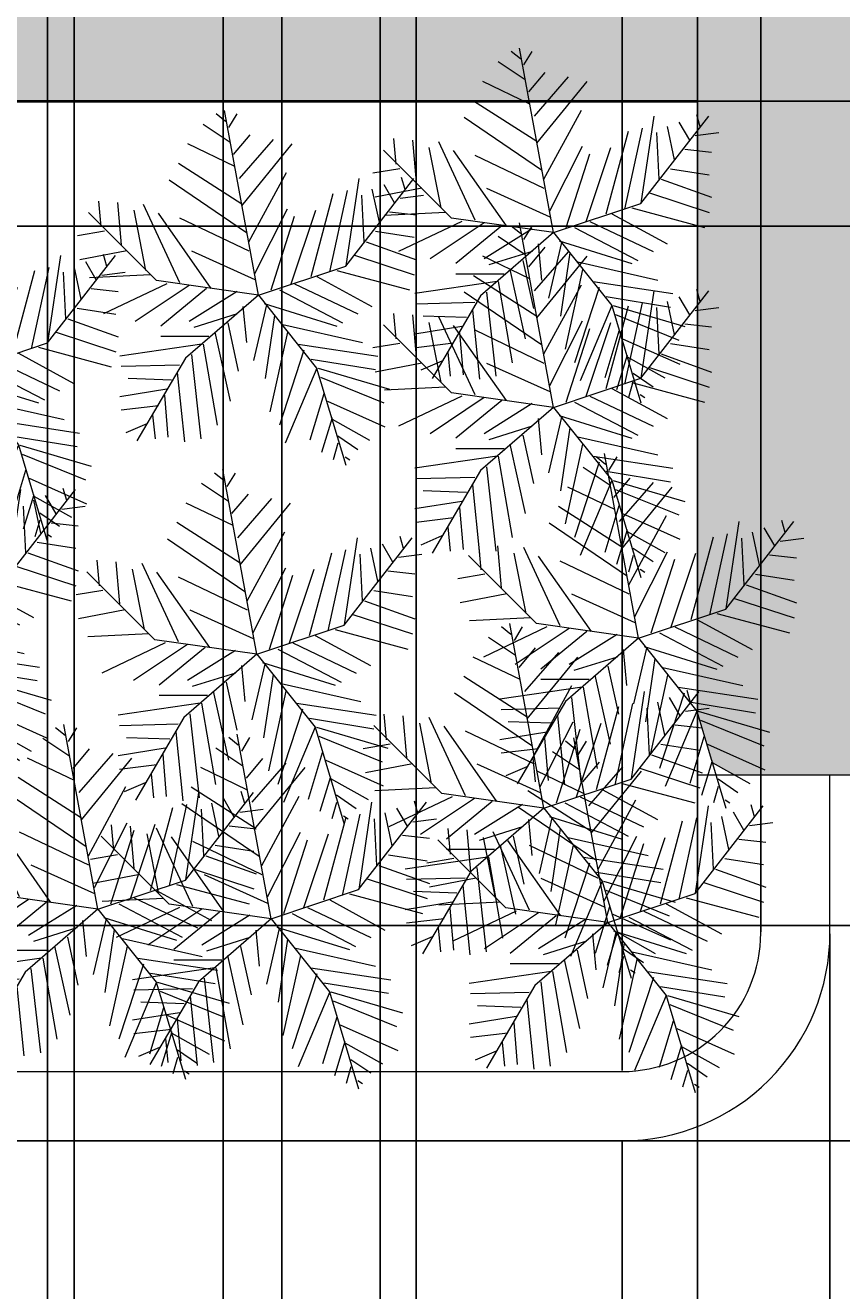
# Model space of a CAD drawing. Units: inches. Extents: x 818 to 1898, y 976 to 2364.
# Tile 40 of 96: x 1667 to 1714, y 1277 to 1350. Entities that reach past the tile are written whole.
import ezdxf

# ---------------------------------------------------------------- set-up
doc = ezdxf.new("R2010")
doc.units = ezdxf.units.IN
doc.header["$LTSCALE"] = 5
doc.header["$MEASUREMENT"] = 0
for name, color, linetype, lineweight in [('A-ANNO-DIMS', 2, 'Continuous', 18), ('A-WALL', 7, 'Continuous', 40), ('L-PLNT-BEDS', 94, 'Continuous', 18)]:
    doc.layers.add(name, color=color, linetype=linetype, lineweight=lineweight)
doc.layers.add('A-WALL-PATT', color=251, linetype='Continuous', lineweight=13, true_color=0x636466)
doc.layers.add('L-PLNT', color=116, linetype='Continuous', lineweight=13, true_color=0x136734)
doc.styles.get("Standard").update_dxf_attribs({"font": 'arial.ttf'})
doc.dimstyles.get("Standard").update_dxf_attribs({"dimtxt": 0.18, "dimasz": 0.18, "dimexe": 0.18, "dimexo": 0.0625, "dimgap": 0.09, "dimtad": 0, "dimtih": 1, "dimtoh": 1, "dimdec": 4, "dimzin": 0, "dimdsep": 46, "dimtxsty": 'Standard', "dimcen": 0.09, "dimadec": 0, "dimazin": 0, "dimtfac": 1, "dimtdec": 4, "dimtofl": 0, "dimtmove": 0, "dimatfit": 3, "dimfxl": 1, "dimtolj": 1, "dimtzin": 0, "dimarcsym": 0})

# ---------------------------------------------------------------- blocks, each defined once
blk = doc.blocks.new('SHRUB-ACCENT')
for p, q in [((10.438, 9.815), (8.475, 20.472)), ((8.533, 19.844), (7.992, 20.278)), ((8.737, 19.496), (9.211, 20.278)), ((8.804, 18.628), (7.247, 19.67)), ((9.008, 17.934), (9.956, 19.062)), ((9.075, 17.239), (6.366, 18.541)), ((9.346, 16.544), (11.31, 18.802)), ((9.482, 14.981), (12.394, 18.541)), ((9.482, 15.068), (5.824, 17.413)), ((9.888, 12.898), (12.055, 16.892)), ((9.753, 13.419), (5.283, 16.458)), ((15.486, 11.498), (19.412, 16.546)), ((15.509, 11.509), (16.254, 16.544)), ((17.677, 16.197), (18.286, 15.155)), ((18.693, 16.631), (18.896, 15.937)), ((13.478, 10.901), (14.764, 15.676)), ((14.561, 11.161), (15.577, 15.85)), ((16.39, 15.589), (16.525, 12.898)), ((16.999, 15.937), (17.406, 14.026)), ((18.625, 15.416), (19.979, 15.589)), ((1.354, 13.766), (1.219, 15.242)), ((2.303, 15.155), (2.506, 12.724)), ((3.251, 14.721), (3.928, 11.248)), ((3.793, 15.068), (5.892, 10.553)), ((10.227, 11.074), (12.123, 14.808)), ((12.326, 10.467), (13.748, 14.721)), ((18.015, 14.634), (19.573, 14.461)), ((4.549, 10.657), (0.623, 14.583)), ((7.721, 10.206), (4.673, 14.547)), ((5.892, 14.287), (9.888, 12.377)), ((11.175, 10.119), (12.529, 14.374)), ((1.558, 13.505), (0, 13.245)), ((17.203, 13.505), (19.437, 13.158)), ((16.661, 12.898), (19.573, 11.856)), ((2.845, 12.377), (0.136, 11.856)), ((6.569, 12.377), (10.227, 10.727)), ((15.983, 12.116), (19.437, 10.988)), ((4.199, 10.988), (0.677, 10.814)), ((10.438, 9.815), (15.486, 11.498)), ((14.968, 11.248), (19.166, 10.119)), ((5.147, 10.467), (1.49, 8.73)), ((6.434, 10.38), (3.319, 8.296)), ((10.438, 9.815), (4.549, 10.657)), ((12.529, 10.467), (16.187, 8.73)), ((13.816, 10.901), (16.999, 9.164)), ((7.45, 10.206), (4.809, 8.035)), ((10.438, 9.815), (6.231, 6.17)), ((9.211, 10.033), (6.434, 8.296)), ((10.438, 9.815), (13.803, 5.609)), ((11.649, 10.119), (15.306, 8.209)), ((9.549, 9.164), (9.753, 7.08)), ((10.904, 9.251), (10.159, 6.039)), ((10.769, 9.338), (14.968, 8.035)), ((9.211, 8.73), (6.705, 7.949)), ((8.669, 8.209), (9.278, 5.431)), ((11.378, 8.643), (10.836, 4.997)), ((11.852, 8.122), (16.457, 7.08)), ((7.585, 7.428), (4.809, 7.428)), ((7.924, 7.688), (8.804, 3.694)), ((12.123, 7.688), (11.107, 3.086)), ((7.179, 6.994), (2.438, 6.299)), ((7.247, 6.994), (8.06, 2.305)), ((13.071, 6.646), (11.649, 2.305)), ((12.733, 6.994), (17.338, 6.299)), ((6.231, 6.17), (3.427, 1.402)), ((6.569, 6.386), (7.111, 1.524)), ((13.478, 6.125), (17.203, 5.517)), ((5.892, 5.778), (2.506, 5.691)), ((5.757, 5.344), (6.163, 1.35)), ((13.816, 5.604), (11.988, 1.263)), ((13.803, 5.609), (15.486, 0)), ((13.884, 5.604), (18.015, 4.389)), ((5.147, 4.389), (2.438, 3.955)), ((5.418, 4.91), (2.912, 4.997)), ((14.019, 5.083), (17.677, 3.607)), ((5.012, 4.041), (5.215, 1.61)), ((14.223, 4.128), (13.41, 1.437)), ((14.426, 3.694), (17.744, 2.218)), ((4.673, 3.434), (2.506, 3.173)), ((3.996, 2.392), (2.777, 1.871)), ((4.334, 2.913), (4.47, 1.524)), ((14.697, 2.739), (14.087, 0.742)), ((14.697, 2.652), (16.864, 1.437)), ((15.035, 1.697), (16.187, 0.916)), ((15.035, 1.263), (14.764, 0.308)), ((15.442, 0.482), (15.712, 0.308))]:
    blk.add_line(p, q)
blk = doc.blocks.new('*D65')
at = {"layer": 'A-ANNO-DIMS', "color": 0, "lineweight": -2, "ltscale": 5, "transparency": 16777216}
for p, q in [((1430.725, 1346.016), (1430.725, 975.663)), ((1714.725, 1346.016), (1714.725, 975.663)), ((1430.905, 975.843), (1572.435, 975.843)), ((1714.545, 975.843), (1573.015, 975.843))]:
    blk.add_line(p, q, dxfattribs=at)
at = {"layer": 'A-ANNO-DIMS', "color": 0, "ltscale": 5, "transparency": 16777216}
for points in [[(1430.905, 975.873), (1430.905, 975.813), (1430.725, 975.843)], [(1714.545, 975.873), (1714.545, 975.813), (1714.725, 975.843)]]:
    blk.add_solid(points, dxfattribs=at)
at = {"layer": 'Defpoints', "color": 0, "ltscale": 5, "transparency": 16777216}
for p in [(1430.725, 1346.078), (1714.725, 1346.078), (1714.725, 975.843)]:
    blk.add_point(p, dxfattribs=at)
at = {"layer": 'A-ANNO-DIMS', "color": 0, "ltscale": 5, "transparency": 16777216, "insert": (1572.725, 975.843), "char_height": 0.18, "attachment_point": 5}
blk.add_mtext('\\A1;284', dxfattribs=at)
blk = doc.blocks.new('*D103')
at = {"layer": 'A-ANNO-DIMS', "color": 0, "lineweight": -2, "ltscale": 5, "transparency": 16777216}
for p, q in [((1626.575, 1071.118), (1626.575, 2363.873)), ((1626.755, 2363.693), (1657.699, 2363.693)), ((1689.291, 2363.693), (1658.348, 2363.693)), ((1689.471, 1071.118), (1689.471, 2363.873))]:
    blk.add_line(p, q, dxfattribs=at)
at = {"layer": 'A-ANNO-DIMS', "color": 0, "ltscale": 5, "transparency": 16777216}
for points in [[(1626.755, 2363.723), (1626.755, 2363.663), (1626.575, 2363.693)], [(1689.291, 2363.723), (1689.291, 2363.663), (1689.471, 2363.693)]]:
    blk.add_solid(points, dxfattribs=at)
at = {"layer": 'Defpoints', "color": 0, "ltscale": 5, "transparency": 16777216}
for p in [(1689.471, 2363.693), (1626.575, 1071.055), (1689.471, 1071.055)]:
    blk.add_point(p, dxfattribs=at)
at = {"layer": 'A-ANNO-DIMS', "color": 0, "ltscale": 5, "transparency": 16777216, "insert": (1658.023, 2363.693), "char_height": 0.18, "attachment_point": 5}
blk.add_mtext('\\A1;62.9', dxfattribs=at)
blk = doc.blocks.new('*D104')
at = {"layer": 'A-ANNO-DIMS', "color": 0, "lineweight": -2, "ltscale": 5, "transparency": 16777216}
for p, q in [((1689.471, 1071.118), (1689.471, 2363.873)), ((1689.651, 2363.693), (1717.401, 2363.693)), ((1745.903, 2363.693), (1718.154, 2363.693)), ((1746.083, 1071.118), (1746.083, 2363.873))]:
    blk.add_line(p, q, dxfattribs=at)
at = {"layer": 'A-ANNO-DIMS', "color": 0, "ltscale": 5, "transparency": 16777216}
for points in [[(1689.651, 2363.723), (1689.651, 2363.663), (1689.471, 2363.693)], [(1745.903, 2363.723), (1745.903, 2363.663), (1746.083, 2363.693)]]:
    blk.add_solid(points, dxfattribs=at)
at = {"layer": 'Defpoints', "color": 0, "ltscale": 5, "transparency": 16777216}
for p in [(1746.083, 2363.693), (1689.471, 1071.055), (1746.083, 1071.055)]:
    blk.add_point(p, dxfattribs=at)
at = {"layer": 'A-ANNO-DIMS', "color": 0, "ltscale": 5, "transparency": 16777216, "insert": (1717.777, 2363.693), "char_height": 0.18, "attachment_point": 5}
blk.add_mtext('\\A1;56.61', dxfattribs=at)
blk = doc.blocks.new('*D113')
at = {"layer": 'A-ANNO-DIMS', "color": 0, "lineweight": -2, "ltscale": 5, "transparency": 16777216}
for p, q in [((1430.788, 1346.078), (1897.916, 1346.078)), ((1897.736, 1345.898), (1897.736, 1316.26)), ((1897.736, 1286.258), (1897.736, 1315.896)), ((1430.788, 1286.078), (1897.916, 1286.078))]:
    blk.add_line(p, q, dxfattribs=at)
at = {"layer": 'A-ANNO-DIMS', "color": 0, "ltscale": 5, "transparency": 16777216}
for points in [[(1897.706, 1345.898), (1897.766, 1345.898), (1897.736, 1346.078)], [(1897.706, 1286.258), (1897.766, 1286.258), (1897.736, 1286.078)]]:
    blk.add_solid(points, dxfattribs=at)
at = {"layer": 'Defpoints', "color": 0, "ltscale": 5, "transparency": 16777216}
for p in [(1430.725, 1346.078), (1897.736, 1346.078), (1430.725, 1286.078)]:
    blk.add_point(p, dxfattribs=at)
at = {"layer": 'A-ANNO-DIMS', "color": 0, "ltscale": 5, "transparency": 16777216, "insert": (1897.736, 1316.078), "char_height": 0.18, "attachment_point": 5}
blk.add_mtext('\\A1;60', dxfattribs=at)
blk = doc.blocks.new('*D115')
at = {"layer": 'A-ANNO-DIMS', "color": 0, "lineweight": -2, "ltscale": 5, "transparency": 16777216}
for p, q in [((1766.29, 1377.656), (818.026, 1377.656)), ((818.206, 1377.476), (818.206, 1338.262)), ((818.206, 1298.684), (818.206, 1337.898)), ((1766.29, 1298.504), (818.026, 1298.504))]:
    blk.add_line(p, q, dxfattribs=at)
at = {"layer": 'A-ANNO-DIMS', "color": 0, "ltscale": 5, "transparency": 16777216}
for points in [[(818.176, 1377.476), (818.236, 1377.476), (818.206, 1377.656)], [(818.176, 1298.684), (818.236, 1298.684), (818.206, 1298.504)]]:
    blk.add_solid(points, dxfattribs=at)
at = {"layer": 'Defpoints', "color": 0, "ltscale": 5, "transparency": 16777216}
for p in [(818.206, 1377.656), (1766.352, 1377.656), (1766.352, 1298.504)]:
    blk.add_point(p, dxfattribs=at)
at = {"layer": 'A-ANNO-DIMS', "color": 0, "ltscale": 5, "transparency": 16777216, "insert": (818.206, 1338.08), "char_height": 0.18, "attachment_point": 5}
blk.add_mtext('\\A1;79.15', dxfattribs=at)
blk = doc.blocks.new('*D153')
at = {"layer": 'A-ANNO-DIMS', "color": 0, "lineweight": -2, "ltscale": 5, "transparency": 16777216}
for p, q in [((1713.369, 1298.016), (1713.369, 975.663)), ((1701.369, 1286.016), (1701.369, 975.663)), ((1701.549, 975.843), (1707.159, 975.843)), ((1713.189, 975.843), (1707.578, 975.843))]:
    blk.add_line(p, q, dxfattribs=at)
at = {"layer": 'A-ANNO-DIMS', "color": 0, "ltscale": 5, "transparency": 16777216}
for points in [[(1701.549, 975.873), (1701.549, 975.813), (1701.369, 975.843)], [(1713.189, 975.873), (1713.189, 975.813), (1713.369, 975.843)]]:
    blk.add_solid(points, dxfattribs=at)
at = {"layer": 'Defpoints', "color": 0, "ltscale": 5, "transparency": 16777216}
for p in [(1713.369, 1298.078), (1701.369, 1286.078), (1713.369, 975.843)]:
    blk.add_point(p, dxfattribs=at)
at = {"layer": 'A-ANNO-DIMS', "color": 0, "ltscale": 5, "transparency": 16777216, "insert": (1707.369, 975.843), "char_height": 0.18, "attachment_point": 5}
blk.add_mtext('\\A1;12', dxfattribs=at)
blk = doc.blocks.new('*D154')
at = {"layer": 'A-ANNO-DIMS', "color": 0, "lineweight": -2, "ltscale": 5, "transparency": 16777216}
for p, q in [((1701.369, 1290.141), (1701.369, 2363.873)), ((1701.549, 2363.693), (1705.22, 2363.693)), ((1709.189, 2363.693), (1705.518, 2363.693)), ((1709.369, 1298.141), (1709.369, 2363.873))]:
    blk.add_line(p, q, dxfattribs=at)
at = {"layer": 'A-ANNO-DIMS', "color": 0, "ltscale": 5, "transparency": 16777216}
for points in [[(1701.549, 2363.723), (1701.549, 2363.663), (1701.369, 2363.693)], [(1709.189, 2363.723), (1709.189, 2363.663), (1709.369, 2363.693)]]:
    blk.add_solid(points, dxfattribs=at)
at = {"layer": 'Defpoints', "color": 0, "ltscale": 5, "transparency": 16777216}
for p in [(1709.369, 2363.693), (1709.369, 1298.078), (1701.369, 1290.078)]:
    blk.add_point(p, dxfattribs=at)
at = {"layer": 'A-ANNO-DIMS', "color": 0, "ltscale": 5, "transparency": 16777216, "insert": (1705.369, 2363.693), "char_height": 0.18, "attachment_point": 5}
blk.add_mtext('\\A1;8', dxfattribs=at)
blk = doc.blocks.new('*D178')
at = {"layer": 'A-ANNO-DIMS', "color": 0, "lineweight": -2, "ltscale": 5, "transparency": 16777216}
for p, q in [((1669.725, 1600.016), (1669.725, 975.663)), ((1705.725, 1600.016), (1705.725, 975.663)), ((1669.905, 975.843), (1687.506, 975.843)), ((1705.545, 975.843), (1687.944, 975.843))]:
    blk.add_line(p, q, dxfattribs=at)
at = {"layer": 'A-ANNO-DIMS', "color": 0, "ltscale": 5, "transparency": 16777216}
for points in [[(1669.905, 975.873), (1669.905, 975.813), (1669.725, 975.843)], [(1705.545, 975.873), (1705.545, 975.813), (1705.725, 975.843)]]:
    blk.add_solid(points, dxfattribs=at)
at = {"layer": 'Defpoints', "color": 0, "ltscale": 5, "transparency": 16777216}
for p in [(1669.725, 1600.078), (1705.725, 1600.078), (1705.725, 975.843)]:
    blk.add_point(p, dxfattribs=at)
at = {"layer": 'A-ANNO-DIMS', "color": 0, "ltscale": 5, "transparency": 16777216, "insert": (1687.725, 975.843), "char_height": 0.18, "attachment_point": 5}
blk.add_mtext('\\A1;36', dxfattribs=at)
blk = doc.blocks.new('*D180')
at = {"layer": 'A-ANNO-DIMS', "color": 0, "lineweight": -2, "ltscale": 5, "transparency": 16777216}
for p, q in [((1599.725, 1639.516), (1599.725, 975.663)), ((1669.725, 1639.516), (1669.725, 975.663)), ((1599.905, 975.843), (1634.507, 975.843)), ((1669.545, 975.843), (1634.943, 975.843))]:
    blk.add_line(p, q, dxfattribs=at)
at = {"layer": 'A-ANNO-DIMS', "color": 0, "ltscale": 5, "transparency": 16777216}
for points in [[(1599.905, 975.873), (1599.905, 975.813), (1599.725, 975.843)], [(1669.545, 975.873), (1669.545, 975.813), (1669.725, 975.843)]]:
    blk.add_solid(points, dxfattribs=at)
at = {"layer": 'Defpoints', "color": 0, "ltscale": 5, "transparency": 16777216}
for p in [(1599.725, 1639.578), (1669.725, 1639.578), (1669.725, 975.843)]:
    blk.add_point(p, dxfattribs=at)
at = {"layer": 'A-ANNO-DIMS', "color": 0, "ltscale": 5, "transparency": 16777216, "insert": (1634.725, 975.843), "char_height": 0.18, "attachment_point": 5}
blk.add_mtext('\\A1;70', dxfattribs=at)
blk = doc.blocks.new('*D193')
at = {"layer": 'A-ANNO-DIMS', "color": 0, "lineweight": -2, "ltscale": 5, "transparency": 16777216}
for p, q in [((1660.377, 1346.078), (1897.916, 1346.078)), ((1897.736, 1345.898), (1897.736, 1342.654)), ((1897.736, 1339.045), (1897.736, 1342.29)), ((1660.377, 1338.865), (1897.916, 1338.865))]:
    blk.add_line(p, q, dxfattribs=at)
at = {"layer": 'A-ANNO-DIMS', "color": 0, "ltscale": 5, "transparency": 16777216}
for points in [[(1897.706, 1345.898), (1897.766, 1345.898), (1897.736, 1346.078)], [(1897.706, 1339.045), (1897.766, 1339.045), (1897.736, 1338.865)]]:
    blk.add_solid(points, dxfattribs=at)
at = {"layer": 'Defpoints', "color": 0, "ltscale": 5, "transparency": 16777216}
for p in [(1660.314, 1346.078), (1897.736, 1346.078), (1660.314, 1338.865)]:
    blk.add_point(p, dxfattribs=at)
at = {"layer": 'A-ANNO-DIMS', "color": 0, "ltscale": 5, "transparency": 16777216, "insert": (1897.736, 1342.472), "char_height": 0.18, "attachment_point": 5}
blk.add_mtext('\\A1;7.213', dxfattribs=at)
blk = doc.blocks.new('*D198')
at = {"layer": 'A-ANNO-DIMS', "color": 0, "lineweight": -2, "ltscale": 5, "transparency": 16777216}
for p, q in [((1741.841, 1545.016), (1741.841, 975.663)), ((1430.725, 1346.016), (1430.725, 975.663)), ((1430.905, 975.843), (1585.907, 975.843)), ((1741.661, 975.843), (1586.659, 975.843))]:
    blk.add_line(p, q, dxfattribs=at)
at = {"layer": 'A-ANNO-DIMS', "color": 0, "ltscale": 5, "transparency": 16777216}
for points in [[(1430.905, 975.873), (1430.905, 975.813), (1430.725, 975.843)], [(1741.661, 975.873), (1741.661, 975.813), (1741.841, 975.843)]]:
    blk.add_solid(points, dxfattribs=at)
at = {"layer": 'Defpoints', "color": 0, "ltscale": 5, "transparency": 16777216}
for p in [(1741.841, 1545.078), (1430.725, 1346.078), (1741.841, 975.843)]:
    blk.add_point(p, dxfattribs=at)
at = {"layer": 'A-ANNO-DIMS', "color": 0, "ltscale": 5, "transparency": 16777216, "insert": (1586.283, 975.843), "char_height": 0.18, "attachment_point": 5}
blk.add_mtext('\\A1;311.1', dxfattribs=at)
blk = doc.blocks.new('*D199')
at = {"layer": 'A-ANNO-DIMS', "color": 0, "lineweight": -2, "ltscale": 5, "transparency": 16777216}
for p, q in [((1559.788, 1687.078), (1897.916, 1687.078)), ((1897.736, 1686.898), (1897.736, 1513.154)), ((1897.736, 1339.045), (1897.736, 1512.79)), ((1660.377, 1338.865), (1897.916, 1338.865))]:
    blk.add_line(p, q, dxfattribs=at)
at = {"layer": 'A-ANNO-DIMS', "color": 0, "ltscale": 5, "transparency": 16777216}
for points in [[(1897.706, 1686.898), (1897.766, 1686.898), (1897.736, 1687.078)], [(1897.706, 1339.045), (1897.766, 1339.045), (1897.736, 1338.865)]]:
    blk.add_solid(points, dxfattribs=at)
at = {"layer": 'Defpoints', "color": 0, "ltscale": 5, "transparency": 16777216}
for p in [(1559.725, 1687.078), (1897.736, 1687.078), (1660.314, 1338.865)]:
    blk.add_point(p, dxfattribs=at)
at = {"layer": 'A-ANNO-DIMS', "color": 0, "ltscale": 5, "transparency": 16777216, "insert": (1897.736, 1512.972), "char_height": 0.18, "attachment_point": 5}
blk.add_mtext('\\A1;348.2', dxfattribs=at)
blk = doc.blocks.new('*D200')
at = {"layer": 'A-ANNO-DIMS', "color": 0, "lineweight": -2, "ltscale": 5, "transparency": 16777216}
for p, q in [((1678.33, 1477.364), (1678.33, 975.663)), ((1705.725, 1477.364), (1705.725, 975.663)), ((1678.51, 975.843), (1691.562, 975.843)), ((1705.545, 975.843), (1692.493, 975.843))]:
    blk.add_line(p, q, dxfattribs=at)
at = {"layer": 'A-ANNO-DIMS', "color": 0, "ltscale": 5, "transparency": 16777216}
for points in [[(1678.51, 975.873), (1678.51, 975.813), (1678.33, 975.843)], [(1705.545, 975.873), (1705.545, 975.813), (1705.725, 975.843)]]:
    blk.add_solid(points, dxfattribs=at)
at = {"layer": 'Defpoints', "color": 0, "ltscale": 5, "transparency": 16777216}
for p in [(1678.33, 1477.426), (1705.725, 1477.426), (1705.725, 975.843)]:
    blk.add_point(p, dxfattribs=at)
at = {"layer": 'A-ANNO-DIMS', "color": 0, "ltscale": 5, "transparency": 16777216, "insert": (1692.028, 975.843), "char_height": 0.18, "attachment_point": 5}
blk.add_mtext('\\A1;27.395', dxfattribs=at)
blk = doc.blocks.new('*D212')
at = {"layer": 'A-ANNO-DIMS', "color": 0, "lineweight": -2, "ltscale": 5, "transparency": 16777216}
for p, q in [((1681.725, 1900.016), (1681.725, 975.663)), ((1705.725, 1876.016), (1705.725, 975.663)), ((1681.905, 975.843), (1693.505, 975.843)), ((1705.545, 975.843), (1693.945, 975.843))]:
    blk.add_line(p, q, dxfattribs=at)
at = {"layer": 'A-ANNO-DIMS', "color": 0, "ltscale": 5, "transparency": 16777216}
for points in [[(1681.905, 975.873), (1681.905, 975.813), (1681.725, 975.843)], [(1705.545, 975.873), (1705.545, 975.813), (1705.725, 975.843)]]:
    blk.add_solid(points, dxfattribs=at)
at = {"layer": 'Defpoints', "color": 0, "ltscale": 5, "transparency": 16777216}
for p in [(1681.725, 1900.078), (1705.725, 1876.078), (1705.725, 975.843)]:
    blk.add_point(p, dxfattribs=at)
at = {"layer": 'A-ANNO-DIMS', "color": 0, "ltscale": 5, "transparency": 16777216, "insert": (1693.725, 975.843), "char_height": 0.18, "attachment_point": 5}
blk.add_mtext('\\A1;24', dxfattribs=at)
blk = doc.blocks.new('*D214')
at = {"layer": 'A-ANNO-DIMS', "color": 0, "lineweight": -2, "ltscale": 5, "transparency": 16777216}
for p, q in [((1511.725, 1687.016), (1511.725, 975.663)), ((1714.725, 1687.016), (1714.725, 975.663)), ((1511.905, 975.843), (1612.935, 975.843)), ((1714.545, 975.843), (1613.516, 975.843))]:
    blk.add_line(p, q, dxfattribs=at)
at = {"layer": 'A-ANNO-DIMS', "color": 0, "ltscale": 5, "transparency": 16777216}
for points in [[(1511.905, 975.873), (1511.905, 975.813), (1511.725, 975.843)], [(1714.545, 975.873), (1714.545, 975.813), (1714.725, 975.843)]]:
    blk.add_solid(points, dxfattribs=at)
at = {"layer": 'Defpoints', "color": 0, "ltscale": 5, "transparency": 16777216}
for p in [(1511.725, 1687.078), (1714.725, 1687.078), (1714.725, 975.843)]:
    blk.add_point(p, dxfattribs=at)
at = {"layer": 'A-ANNO-DIMS', "color": 0, "ltscale": 5, "transparency": 16777216, "insert": (1613.225, 975.843), "char_height": 0.18, "attachment_point": 5}
blk.add_mtext('\\A1;203', dxfattribs=at)
blk = doc.blocks.new('*D221')
at = {"layer": 'A-ANNO-DIMS', "color": 0, "lineweight": -2, "ltscale": 5, "transparency": 16777216}
for p, q in [((1668.184, 1696.016), (1668.184, 975.663)), ((1705.725, 1696.016), (1705.725, 975.663)), ((1668.364, 975.843), (1686.561, 975.843)), ((1705.545, 975.843), (1687.348, 975.843))]:
    blk.add_line(p, q, dxfattribs=at)
at = {"layer": 'A-ANNO-DIMS', "color": 0, "ltscale": 5, "transparency": 16777216}
for points in [[(1668.364, 975.873), (1668.364, 975.813), (1668.184, 975.843)], [(1705.545, 975.873), (1705.545, 975.813), (1705.725, 975.843)]]:
    blk.add_solid(points, dxfattribs=at)
at = {"layer": 'Defpoints', "color": 0, "ltscale": 5, "transparency": 16777216}
for p in [(1668.184, 1696.078), (1705.725, 1696.078), (1705.725, 975.843)]:
    blk.add_point(p, dxfattribs=at)
at = {"layer": 'A-ANNO-DIMS', "color": 0, "ltscale": 5, "transparency": 16777216, "insert": (1686.955, 975.843), "char_height": 0.18, "attachment_point": 5}
blk.add_mtext('\\A1;37.54', dxfattribs=at)
blk = doc.blocks.new('*D228')
at = {"layer": 'A-ANNO-DIMS', "color": 0, "lineweight": -2, "ltscale": 5, "transparency": 16777216}
for p, q in [((1687.394, 1802.016), (1687.394, 975.663)), ((1705.725, 1802.016), (1705.725, 975.663)), ((1687.574, 975.843), (1696.174, 975.843)), ((1705.545, 975.843), (1696.945, 975.843))]:
    blk.add_line(p, q, dxfattribs=at)
at = {"layer": 'A-ANNO-DIMS', "color": 0, "ltscale": 5, "transparency": 16777216}
for points in [[(1687.574, 975.873), (1687.574, 975.813), (1687.394, 975.843)], [(1705.545, 975.873), (1705.545, 975.813), (1705.725, 975.843)]]:
    blk.add_solid(points, dxfattribs=at)
at = {"layer": 'Defpoints', "color": 0, "ltscale": 5, "transparency": 16777216}
for p in [(1687.394, 1802.078), (1705.725, 1802.078), (1705.725, 975.843)]:
    blk.add_point(p, dxfattribs=at)
at = {"layer": 'A-ANNO-DIMS', "color": 0, "ltscale": 5, "transparency": 16777216, "insert": (1696.56, 975.843), "char_height": 0.18, "attachment_point": 5}
blk.add_mtext('\\A1;18.33', dxfattribs=at)

msp = doc.modelspace()

# ---------------------------------------------------------------- hatches: boundary and pattern name
at = {"layer": 'A-WALL-PATT', "ltscale": 5}
h = msp.add_hatch(color=256, dxfattribs=at)
h.dxf.hatch_style = 1
h.paths.add_polyline_path([(1714.7251, 1521.0782), (1705.7251, 1521.0782), (1705.7251, 1467.0782), (1654.7252, 1467.0782), (1654.7252, 1463.0782), (1705.7251, 1463.0782), (1705.7251, 1355.0782), (1622.7252, 1355.0782), (1622.7252, 1379.0782), (1622.7252, 1386.6857), (1616.7252, 1386.6857), (1616.7252, 1355.0782), (1490.9163, 1355.0782), (1490.9163, 1346.0782), (1544.7605, 1346.0782), (1544.6132, 1346.8783), (1544.6729, 1346.84), (1544.6299, 1346.7874), (1544.7605, 1346.0782), (1555.1299, 1346.0782), (1555.1299, 1341.5528), (1556.1599, 1340.8639), (1556.5281, 1338.8654), (1660.3141, 1338.8654), (1660.3141, 1346.0782), (1705.7251, 1346.0782), (1705.7251, 1345.0768), (1705.8704, 1344.58), (1705.7251, 1344.3933), (1705.7251, 1334.9904), (1705.8704, 1334.4936), (1705.7251, 1334.3068), (1705.7251, 1316.2253), (1707.3573, 1316.7694), (1707.3847, 1316.8046), (1707.3807, 1316.7771), (1705.7251, 1316.2253), (1705.7251, 1314.1392), (1705.7251, 1312.0957), (1705.8703, 1312.0739), (1705.7251, 1311.8873), (1705.7251, 1310.7121), (1706.5603, 1307.9282), (1707.8887, 1307.1831), (1714.7251, 1307.1831), (1714.7251, 1346.0782)])

# ---------------------------------------------------------------- linework, layer by layer
at = {"layer": 'A-WALL'}
msp.add_line((1660.3141, 1346.0782), (1705.7251, 1346.0782), dxfattribs=at)
at = {"layer": 'L-PLNT'}
for p, q in [((1697.4011, 1338.4984), (1695.438, 1349.1549)), ((1695.7676, 1347.3112), (1694.2099, 1348.3531)), ((1695.4967, 1348.5268), (1694.9549, 1348.9609)), ((1695.6999, 1348.1794), (1696.1741, 1348.9609)), ((1695.9708, 1346.6166), (1696.9191, 1347.7453)), ((1696.0385, 1345.9219), (1693.3295, 1347.2242)), ((1696.3094, 1345.2273), (1698.2736, 1347.4848)), ((1696.445, 1343.6644), (1699.3572, 1347.2242)), ((1696.445, 1343.7513), (1692.7877, 1346.0956)), ((1696.8512, 1341.5805), (1699.0186, 1345.5747)), ((1696.7159, 1342.1016), (1692.2459, 1345.1404)), ((1702.4489, 1340.181), (1706.375, 1345.2288)), ((1702.4727, 1340.1914), (1703.2177, 1345.2273)), ((1704.6399, 1344.88), (1705.2494, 1343.8381)), ((1705.6558, 1345.3141), (1705.8588, 1344.6195)), ((1700.4408, 1339.5836), (1701.7276, 1344.3591)), ((1701.5244, 1339.8441), (1702.5403, 1344.5328)), ((1703.353, 1344.2722), (1703.4886, 1341.5805)), ((1703.9625, 1344.6195), (1704.369, 1342.7094)), ((1705.5881, 1344.0985), (1706.9426, 1344.2722)), ((1691.5119, 1339.3397), (1687.5858, 1343.2658)), ((1688.3177, 1342.449), (1688.1824, 1343.925)), ((1689.266, 1343.8381), (1689.469, 1341.407)), ((1690.214, 1343.4039), (1690.8914, 1339.931)), ((1690.7558, 1343.7513), (1692.8554, 1339.2363)), ((1694.684, 1338.8891), (1691.6364, 1343.2303)), ((1697.19, 1339.7573), (1699.0863, 1343.4909)), ((1699.2895, 1339.1495), (1700.7117, 1343.4039)), ((1704.9785, 1343.3172), (1706.5362, 1343.1435)), ((1692.8554, 1342.9698), (1696.8512, 1341.0597)), ((1698.138, 1338.8022), (1699.4926, 1343.0566)), ((1688.521, 1342.1883), (1686.9632, 1341.9279)), ((1704.1657, 1342.1883), (1706.4006, 1341.8412)), ((1689.8078, 1341.0597), (1687.0988, 1340.5386)), ((1693.5327, 1341.0597), (1697.19, 1339.41)), ((1703.6239, 1341.5805), (1706.5362, 1340.5386)), ((1702.9466, 1340.7992), (1706.4006, 1339.6704)), ((1691.1623, 1339.6704), (1687.6406, 1339.4967)), ((1697.4011, 1338.4984), (1702.4489, 1340.181)), ((1700.7794, 1339.5836), (1703.9625, 1337.8472)), ((1701.9309, 1339.931), (1706.1297, 1338.8022)), ((1692.1104, 1339.1495), (1688.4533, 1337.4131)), ((1693.3972, 1339.0626), (1690.2819, 1336.9788)), ((1697.4011, 1338.4984), (1691.5119, 1339.3397)), ((1694.4131, 1338.8891), (1691.7718, 1336.7183)), ((1695.4967, 1338.4403), (1694.9549, 1338.8744)), ((1697.4011, 1328.4119), (1695.438, 1339.0685)), ((1695.6999, 1338.093), (1696.1741, 1338.8744)), ((1699.4926, 1339.1495), (1703.1498, 1337.4131)), ((1697.4011, 1338.4984), (1693.1945, 1334.8527)), ((1696.1741, 1338.7154), (1693.3972, 1336.9788)), ((1695.7676, 1337.2247), (1694.2099, 1338.2666)), ((1697.4011, 1338.4984), (1700.7663, 1334.2918)), ((1698.6122, 1338.8022), (1702.2694, 1336.892)), ((1696.1741, 1337.4131), (1693.6681, 1336.6316)), ((1695.9708, 1336.5302), (1696.9191, 1337.6588)), ((1696.3094, 1335.1409), (1698.2736, 1337.3984)), ((1696.5126, 1337.8472), (1696.7159, 1335.7634)), ((1697.8671, 1337.9339), (1697.1223, 1334.7214)), ((1697.7318, 1338.0207), (1701.9309, 1336.7183)), ((1696.0385, 1335.8355), (1693.3295, 1337.1378)), ((1695.6323, 1336.892), (1696.2417, 1334.1136)), ((1696.445, 1333.5779), (1699.3572, 1337.1378)), ((1698.3413, 1337.3261), (1697.7995, 1333.6795)), ((1698.8154, 1336.8053), (1703.4207, 1335.7634)), ((1694.5487, 1336.1105), (1691.7718, 1336.1105)), ((1696.445, 1333.6649), (1692.7877, 1336.0091)), ((1694.8872, 1336.3712), (1695.7676, 1332.3772)), ((1699.0863, 1336.3712), (1698.0704, 1331.7694)), ((1694.1422, 1335.6764), (1689.4013, 1334.9819)), ((1694.2099, 1335.6764), (1695.0228, 1330.9879)), ((1696.8512, 1331.4941), (1699.0186, 1335.4883)), ((1700.0344, 1335.3292), (1698.6122, 1330.9879)), ((1699.6958, 1335.6764), (1704.3011, 1334.9819)), ((1705.6558, 1335.2277), (1705.8588, 1334.5331)), ((1692.8554, 1334.4608), (1689.469, 1334.3741)), ((1693.1945, 1334.8527), (1690.3902, 1330.0853)), ((1696.7159, 1332.0152), (1692.2459, 1335.054)), ((1693.5327, 1335.0686), (1694.0745, 1330.2064)), ((1700.4408, 1334.8082), (1704.1657, 1334.2004)), ((1701.5244, 1329.7576), (1702.5403, 1334.4464)), ((1702.4489, 1330.0945), (1706.375, 1335.1424)), ((1702.4727, 1330.105), (1703.2177, 1335.1409)), ((1703.9625, 1334.5331), (1704.369, 1332.623)), ((1704.6399, 1334.7935), (1705.2494, 1333.7516)), ((1688.3177, 1332.3625), (1688.1824, 1333.8386)), ((1689.266, 1333.7516), (1689.469, 1331.3206)), ((1692.72, 1334.0267), (1693.1263, 1330.0327)), ((1700.7794, 1334.2873), (1698.9508, 1329.946)), ((1700.4408, 1329.4972), (1701.7276, 1334.2727)), ((1700.7663, 1334.2918), (1702.4489, 1328.6831)), ((1700.8473, 1334.2873), (1704.9785, 1333.0717)), ((1700.9826, 1333.7663), (1704.6399, 1332.2902)), ((1703.353, 1334.1857), (1703.4886, 1331.4941)), ((1705.5881, 1334.0121), (1706.9426, 1334.1857)), ((1691.5119, 1329.2532), (1687.5858, 1333.1793)), ((1692.1104, 1333.0717), (1689.4013, 1332.6376)), ((1692.3814, 1333.5926), (1689.8755, 1333.6795)), ((1690.214, 1333.3175), (1690.8914, 1329.8446)), ((1690.7558, 1333.6649), (1692.8554, 1329.1499)), ((1694.684, 1328.8027), (1691.6364, 1333.1438)), ((1697.19, 1329.6709), (1699.0863, 1333.4044)), ((1698.138, 1328.7157), (1699.4926, 1332.9701)), ((1699.2895, 1329.0631), (1700.7117, 1333.3175)), ((1704.9785, 1333.2308), (1706.5362, 1333.0571)), ((1691.975, 1332.7244), (1692.1782, 1330.2934)), ((1692.8554, 1332.8834), (1696.8512, 1330.9732)), ((1701.1858, 1332.8113), (1700.3731, 1330.1197)), ((1701.3891, 1332.3772), (1704.7075, 1330.9012)), ((1688.521, 1332.1019), (1686.9632, 1331.8415)), ((1691.6364, 1332.1166), (1689.469, 1331.8561)), ((1691.2976, 1331.5957), (1691.4332, 1330.2064)), ((1704.1657, 1332.1019), (1706.4006, 1331.7547)), ((1689.8078, 1330.9732), (1687.0988, 1330.4522)), ((1690.9591, 1331.0746), (1689.7399, 1330.5538)), ((1693.5327, 1330.9732), (1697.19, 1329.3235)), ((1701.66, 1331.422), (1701.0503, 1329.4249)), ((1701.66, 1331.3353), (1703.8272, 1330.1197)), ((1703.6239, 1331.4941), (1706.5362, 1330.4522)), ((1697.4011, 1328.4119), (1702.4489, 1330.0945)), ((1701.9985, 1330.3801), (1703.1498, 1329.5986)), ((1702.9466, 1330.7128), (1706.4006, 1329.584)), ((1691.1623, 1329.584), (1687.6406, 1329.4103)), ((1700.7794, 1329.4972), (1703.9625, 1327.7608)), ((1701.9985, 1329.946), (1701.7276, 1328.9908)), ((1701.9309, 1329.8446), (1706.1297, 1328.7157)), ((1692.1104, 1329.0631), (1688.4533, 1327.3266)), ((1693.3972, 1328.9762), (1690.2819, 1326.8923)), ((1697.4011, 1328.4119), (1691.5119, 1329.2532)), ((1694.4131, 1328.8027), (1691.7718, 1326.6319)), ((1696.1741, 1328.629), (1693.3972, 1326.8923)), ((1698.6122, 1328.7157), (1702.2694, 1326.8056)), ((1699.4926, 1329.0631), (1703.1498, 1327.3266)), ((1702.4048, 1329.1645), (1702.6757, 1328.9908)), ((1697.4011, 1328.4119), (1693.1945, 1324.7663)), ((1697.4011, 1328.4119), (1700.7663, 1324.2054)), ((1697.7318, 1327.9343), (1701.9309, 1326.6319)), ((1696.1741, 1327.3266), (1693.6681, 1326.5452)), ((1696.5126, 1327.7608), (1696.7159, 1325.6769)), ((1697.8671, 1327.8475), (1697.1223, 1324.635)), ((1698.3413, 1327.2397), (1697.7995, 1323.5931)), ((1695.6323, 1326.8056), (1696.2417, 1324.0272)), ((1698.8154, 1326.7188), (1703.4207, 1325.6769)), ((1694.5487, 1326.0241), (1691.7718, 1326.0241)), ((1694.8872, 1326.2847), (1695.7676, 1322.2908)), ((1699.0863, 1326.2847), (1698.0704, 1321.683)), ((1702.3095, 1315.0867), (1700.3464, 1325.7433)), ((1694.1422, 1325.59), (1689.4013, 1324.8954)), ((1693.5327, 1324.9822), (1694.0745, 1320.12)), ((1694.2099, 1325.59), (1695.0228, 1320.9015)), ((1700.0344, 1325.2428), (1698.6122, 1320.9015)), ((1700.676, 1323.8995), (1699.1183, 1324.9415)), ((1699.6958, 1325.59), (1704.3011, 1324.8954)), ((1700.4051, 1325.1151), (1699.8633, 1325.5493)), ((1700.6084, 1324.7678), (1701.0825, 1325.5493)), ((1692.8554, 1324.3744), (1689.469, 1324.2876)), ((1693.1945, 1324.7663), (1690.3902, 1319.9988)), ((1700.4408, 1324.7218), (1704.1657, 1324.114)), ((1700.7663, 1324.2054), (1702.4489, 1318.5967)), ((1700.8793, 1323.205), (1701.8275, 1324.3337)), ((1692.3814, 1323.5062), (1689.8755, 1323.5931)), ((1692.72, 1323.9403), (1693.1263, 1319.9463)), ((1700.9469, 1322.5103), (1698.2379, 1323.8126)), ((1700.7794, 1324.2009), (1698.9508, 1319.8596)), ((1700.8473, 1324.2009), (1704.9785, 1322.9853)), ((1700.9826, 1323.6798), (1704.6399, 1322.2038)), ((1701.2178, 1321.8157), (1703.182, 1324.0732)), ((1701.3534, 1320.2527), (1704.2656, 1323.8126)), ((1692.1104, 1322.9853), (1689.4013, 1322.5512)), ((1691.6364, 1322.0301), (1689.469, 1321.7697)), ((1691.975, 1322.6379), (1692.1782, 1320.2069)), ((1701.3534, 1320.3397), (1697.6961, 1322.6839)), ((1701.1858, 1322.7249), (1700.3731, 1320.0332)), ((1701.3891, 1322.2908), (1704.7075, 1320.8147)), ((1701.7596, 1318.1689), (1703.927, 1322.1631)), ((1691.2976, 1321.5093), (1691.4332, 1320.12)), ((1701.6243, 1318.69), (1697.1543, 1321.7288)), ((1701.66, 1321.3356), (1701.0503, 1319.3385)), ((1707.3573, 1316.7694), (1711.2834, 1321.8172)), ((1707.3811, 1316.7798), (1708.1261, 1321.8157)), ((1709.5483, 1321.4683), (1710.1578, 1320.4264)), ((1710.5642, 1321.9025), (1710.7673, 1321.2079)), ((1690.9591, 1320.9882), (1689.7399, 1320.4674)), ((1701.66, 1321.2488), (1703.8272, 1320.0332)), ((1705.3492, 1316.172), (1706.6361, 1320.9475)), ((1706.4328, 1316.4325), (1707.4488, 1321.1212)), ((1708.2615, 1320.8605), (1708.397, 1318.1689)), ((1708.8709, 1321.2079), (1709.2774, 1319.2978)), ((1710.4965, 1320.6869), (1711.8511, 1320.8605)), ((1696.4203, 1315.928), (1692.4942, 1319.8542)), ((1693.2262, 1319.0373), (1693.0908, 1320.5134)), ((1694.1744, 1320.4264), (1694.3774, 1317.9954)), ((1695.1225, 1319.9923), (1695.7998, 1316.5194)), ((1695.6643, 1320.3397), (1697.7638, 1315.8247)), ((1701.9985, 1319.8596), (1701.7276, 1318.9044)), ((1701.9985, 1320.2937), (1703.1498, 1319.5122)), ((1702.0984, 1316.3457), (1703.9947, 1320.0793)), ((1704.1979, 1315.7379), (1705.6201, 1319.9923)), ((1709.8869, 1319.9056), (1711.4446, 1319.7319)), ((1699.5924, 1315.4775), (1696.5448, 1319.8186)), ((1697.7638, 1319.5582), (1701.7596, 1317.6481)), ((1703.0465, 1315.3905), (1704.401, 1319.6449)), ((1693.4294, 1318.7767), (1691.8716, 1318.5163)), ((1702.4048, 1319.0781), (1702.6757, 1318.9044)), ((1709.0742, 1318.7767), (1711.3091, 1318.4295)), ((1694.7162, 1317.6481), (1692.0072, 1317.127)), ((1698.4411, 1317.6481), (1702.0984, 1315.9983)), ((1708.5324, 1318.1689), (1711.4446, 1317.127)), ((1707.855, 1317.3876), (1711.3091, 1316.2588)), ((1696.0707, 1316.2588), (1692.549, 1316.0851)), ((1702.3095, 1315.0867), (1707.3573, 1316.7694)), ((1705.6878, 1316.172), (1708.8709, 1314.4356)), ((1706.8393, 1316.5194), (1711.0382, 1315.3905)), ((1697.0188, 1315.7379), (1693.3617, 1314.0014)), ((1694.941, 1315.3063), (1694.3992, 1315.7404)), ((1696.8454, 1305.2779), (1694.8823, 1315.9345)), ((1695.1443, 1314.9589), (1695.6184, 1315.7404)), ((1698.3056, 1315.651), (1695.1903, 1313.5671)), ((1702.3095, 1315.0867), (1696.4203, 1315.928)), ((1699.3215, 1315.4775), (1696.6802, 1313.3067)), ((1704.401, 1315.7379), (1708.0582, 1314.0014)), ((1695.2119, 1314.0907), (1693.6542, 1315.1326)), ((1702.3095, 1315.0867), (1698.1029, 1311.4411)), ((1701.0825, 1315.3038), (1698.3056, 1313.5671)), ((1702.3095, 1315.0867), (1705.6747, 1310.8802)), ((1703.5206, 1315.3905), (1707.1779, 1313.4804)), ((1695.4828, 1312.7014), (1692.7738, 1314.0038)), ((1695.4152, 1313.3962), (1696.3634, 1314.5248)), ((1695.7537, 1312.0069), (1697.7179, 1314.2644)), ((1695.8893, 1310.4439), (1698.8015, 1314.0038)), ((1701.0825, 1314.0014), (1698.5765, 1313.22)), ((1701.4211, 1314.4356), (1701.6243, 1312.3517)), ((1702.7756, 1314.5223), (1702.0307, 1311.3098)), ((1702.6402, 1314.6091), (1706.8393, 1313.3067)), ((1700.5407, 1313.4804), (1701.1502, 1310.702)), ((1703.2497, 1313.9145), (1702.7079, 1310.2679)), ((1703.7238, 1313.3937), (1708.3291, 1312.3517)), ((1695.8893, 1310.5309), (1692.232, 1312.8751)), ((1699.4571, 1312.6989), (1696.6802, 1312.6989)), ((1699.7957, 1312.9595), (1700.676, 1308.9656)), ((1703.9947, 1312.9595), (1702.9788, 1308.3578)), ((1696.1602, 1308.8811), (1691.6902, 1311.92)), ((1699.0506, 1312.2648), (1694.3098, 1311.5703)), ((1696.2955, 1308.3601), (1698.4629, 1312.3543)), ((1699.1183, 1312.2648), (1699.9312, 1307.5763)), ((1701.8932, 1306.9605), (1705.8193, 1312.0084)), ((1701.917, 1306.971), (1702.662, 1312.0069)), ((1704.9428, 1311.9176), (1703.5206, 1307.5763)), ((1704.6042, 1312.2648), (1709.2095, 1311.5703)), ((1705.1001, 1312.0936), (1705.3031, 1311.3991)), ((1698.1029, 1311.4411), (1695.2986, 1306.6737)), ((1698.4411, 1311.657), (1698.983, 1306.7948)), ((1699.8851, 1306.3632), (1701.1719, 1311.1387)), ((1700.9687, 1306.6236), (1701.9847, 1311.3123)), ((1703.4068, 1311.3991), (1703.8133, 1309.4889)), ((1704.0842, 1311.6595), (1704.6937, 1310.6176)), ((1705.3492, 1311.3966), (1709.0742, 1310.7888)), ((1687.762, 1309.2285), (1687.6267, 1310.7045)), ((1688.7103, 1310.6176), (1688.9133, 1308.1866)), ((1690.2002, 1310.5309), (1692.2997, 1306.0158)), ((1697.7638, 1311.0492), (1694.3774, 1310.9625)), ((1697.6284, 1310.6151), (1698.0347, 1306.6211)), ((1702.7974, 1311.0517), (1702.9329, 1308.3601)), ((1705.6878, 1310.8757), (1703.8592, 1306.5344)), ((1705.0324, 1310.878), (1706.3869, 1311.0517)), ((1705.6747, 1310.8802), (1707.3573, 1305.2715)), ((1705.7557, 1310.8757), (1709.8869, 1309.6601)), ((1705.891, 1310.3547), (1709.5483, 1308.8786)), ((1690.9562, 1306.1192), (1687.0301, 1310.0453)), ((1689.6584, 1310.1835), (1690.3357, 1306.7106)), ((1694.1283, 1305.6687), (1691.0807, 1310.0098)), ((1692.2997, 1309.7494), (1696.2955, 1307.8392)), ((1697.0188, 1309.6601), (1694.3098, 1309.226)), ((1697.2899, 1310.181), (1694.7839, 1310.2679)), ((1696.6343, 1306.5369), (1698.5306, 1310.2704)), ((1697.5824, 1305.5817), (1698.9369, 1309.8361)), ((1698.7338, 1305.9291), (1700.156, 1310.1835)), ((1704.4228, 1310.0967), (1705.9805, 1309.9231)), ((1687.9653, 1308.9679), (1686.4075, 1308.7075)), ((1696.8834, 1309.3127), (1697.0866, 1306.8817)), ((1703.6101, 1308.9679), (1705.845, 1308.6207)), ((1706.0943, 1309.3997), (1705.2816, 1306.7081)), ((1706.2975, 1308.9656), (1709.616, 1307.4895)), ((1696.5448, 1308.7049), (1694.3774, 1308.4445)), ((1696.2061, 1308.1841), (1696.3416, 1306.7948)), ((1703.0683, 1308.3601), (1705.9805, 1307.3182)), ((1689.2521, 1307.8392), (1686.5431, 1307.3182)), ((1692.977, 1307.8392), (1696.6343, 1306.1895)), ((1695.8675, 1307.663), (1694.6483, 1307.1422)), ((1702.3909, 1307.5788), (1705.845, 1306.45)), ((1706.5684, 1308.0104), (1705.9587, 1306.0133)), ((1706.5684, 1307.9236), (1708.7356, 1306.7081)), ((1696.8454, 1305.2779), (1701.8932, 1306.9605)), ((1701.3752, 1306.7106), (1705.5741, 1305.5817)), ((1706.907, 1306.9685), (1708.0582, 1306.187)), ((1690.6066, 1306.45), (1687.0849, 1306.2763)), ((1696.8454, 1305.2779), (1690.9562, 1306.1192)), ((1700.2237, 1306.3632), (1703.4068, 1304.6267)), ((1706.907, 1306.5344), (1706.6361, 1305.5792)), ((1691.5547, 1305.9291), (1687.8976, 1304.1926)), ((1692.8415, 1305.8422), (1689.7262, 1303.7583)), ((1693.8574, 1305.6687), (1691.2161, 1303.4979)), ((1696.8454, 1305.2779), (1692.6388, 1301.6322)), ((1695.6184, 1305.495), (1692.8415, 1303.7583)), ((1696.8454, 1305.2779), (1700.2106, 1301.0714)), ((1698.0565, 1305.5817), (1701.7138, 1303.6716)), ((1698.9369, 1305.9291), (1702.5941, 1304.1926)), ((1707.3132, 1305.7529), (1707.5841, 1305.5792)), ((1695.957, 1304.6267), (1696.1602, 1302.5429)), ((1697.3115, 1304.7135), (1696.5666, 1301.501)), ((1697.1761, 1304.8002), (1701.3752, 1303.4979)), ((1695.6184, 1304.1926), (1693.1124, 1303.4111)), ((1697.7856, 1304.1057), (1697.2438, 1300.4591)), ((1694.3315, 1303.1507), (1695.2119, 1299.1567)), ((1695.0766, 1303.6716), (1695.6861, 1300.8932)), ((1698.5306, 1303.1507), (1697.5147, 1298.5489)), ((1698.2597, 1303.5848), (1702.865, 1302.5429)), ((1693.5865, 1302.456), (1688.8457, 1301.7614)), ((1693.993, 1302.8901), (1691.2161, 1302.8901)), ((1693.6542, 1302.456), (1694.4671, 1297.7675)), ((1699.1401, 1302.456), (1703.7454, 1301.7614)), ((1692.6388, 1301.6322), (1689.8345, 1296.8648)), ((1692.977, 1301.8482), (1693.5188, 1296.986)), ((1699.4787, 1302.1088), (1698.0565, 1297.7675)), ((1699.8851, 1301.5877), (1703.6101, 1300.9799)), ((1692.2997, 1301.2404), (1688.9133, 1301.1536)), ((1700.2237, 1301.0669), (1698.3951, 1296.7255)), ((1700.2106, 1301.0714), (1701.8932, 1295.4626)), ((1700.2916, 1301.0669), (1704.4228, 1299.8513)), ((1691.8258, 1300.3721), (1689.3198, 1300.4591)), ((1692.1643, 1300.8063), (1692.5706, 1296.8123)), ((1700.4269, 1300.5458), (1704.0842, 1299.0698)), ((1691.5547, 1299.8513), (1688.8457, 1299.4172)), ((1691.4193, 1299.5039), (1691.6225, 1297.0729)), ((1700.6301, 1299.5909), (1699.8174, 1296.8992)), ((1691.0807, 1298.8961), (1688.9133, 1298.6357)), ((1700.8334, 1299.1567), (1704.1519, 1297.6807)), ((1690.742, 1298.3753), (1690.8775, 1296.986)), ((1701.1043, 1298.2016), (1700.4946, 1296.2045)), ((1701.1043, 1298.1148), (1703.2715, 1296.8992)), ((1690.4034, 1297.8542), (1689.1842, 1297.3333)), ((1701.4429, 1296.7255), (1701.1719, 1295.7704)), ((1701.4429, 1297.1597), (1702.5941, 1296.3782)), ((1701.8491, 1295.9441), (1702.12, 1295.7704))]:
    msp.add_line(p, q, dxfattribs=at)
at = {"layer": 'L-PLNT-BEDS', "ltscale": 5}
for p, q in [((1705.7251, 1346.0782), (1705.7251, 1314.1392)), ((1705.7251, 1314.1392), (1705.7251, 1307.1831)), ((1714.7251, 1307.1831), (1705.7251, 1307.1831))]:
    msp.add_line(p, q, dxfattribs=at)
for points in [[(1430.7251, 1286.0782), (1701.3688, 1286.0782, 0.4142136), (1713.3688, 1298.0782), (1713.3688, 1307.1831)], [(1430.7251, 1290.0782), (1701.3688, 1290.0782, 0.4142136), (1709.3688, 1298.0782), (1709.3688, 1307.1831)]]:
    msp.add_lwpolyline(points, format="xyb", dxfattribs=at)

# ---------------------------------------------------------------- block references
at = {"layer": 'L-PLNT'}
for p in [(1669.9226, 1325.074), (1652.6968, 1320.6323), (1650.3815, 1307.122), (1669.83, 1304.3459), (1660.6615, 1289.6327), (1670.6635, 1289.0775), (1690.0986, 1288.8637)]:
    msp.add_blockref('SHRUB-ACCENT', p, dxfattribs=at)

# ---------------------------------------------------------------- dimensions: what is measured, and where the dimension line sits
at = {"layer": 'A-ANNO-DIMS', "ltscale": 5}
for base, p1, p2, override, picture, middle in [((1689.4714, 2363.6929), (1626.5748, 1071.0552), (1689.4714, 1071.0552), {"dimdec": 1, "dimlfac": 1, "dimrnd": 0, "dimzin": 0, "dimdsep": 46, "dimlunit": 2}, '*D103', (1658.0231, 2363.6929)), ((1746.0831, 2363.6929), (1689.4714, 1071.0552), (1746.0831, 1071.0552), {"dimdec": 2, "dimlfac": 1, "dimrnd": 0, "dimzin": 0, "dimdsep": 46, "dimlunit": 2}, '*D104', (1717.7772, 2363.6929)), ((1709.3688, 2363.6929), (1701.3688, 1290.0782), (1709.3688, 1298.0782), {"dimdec": 0, "dimlfac": 1, "dimrnd": 0, "dimzin": 0, "dimdsep": 46, "dimlunit": 2}, '*D154', (1705.3688, 2363.6929)), ((1705.7251, 975.8433), (1681.7251, 1900.0782), (1705.7251, 1876.0782), {"dimdec": 0, "dimlfac": 1, "dimrnd": 0, "dimzin": 0, "dimdsep": 46, "dimlunit": 2}, '*D212', (1693.7251, 975.8433)), ((1705.7251, 975.8433), (1687.394, 1802.0782), (1705.7251, 1802.0782), {"dimdec": 2, "dimlfac": 1, "dimrnd": 0, "dimzin": 0, "dimdsep": 46, "dimlunit": 2}, '*D228', (1696.5596, 975.8433)), ((1705.7251, 975.8433), (1668.1841, 1696.0782), (1705.7251, 1696.0782), {"dimdec": 2, "dimlfac": 1, "dimrnd": 0, "dimzin": 0, "dimdsep": 46, "dimlunit": 2}, '*D221', (1686.9546, 975.8433)), ((1714.7251, 975.8433), (1511.7251, 1687.0782), (1714.7251, 1687.0782), {"dimdec": 0, "dimlfac": 1, "dimrnd": 0, "dimzin": 0, "dimdsep": 46, "dimlunit": 2}, '*D214', (1613.2251, 975.8433)), ((1669.7251, 975.8433), (1599.7251, 1639.5782), (1669.7251, 1639.5782), {"dimdec": 0, "dimlfac": 1, "dimrnd": 0, "dimzin": 0, "dimdsep": 46, "dimlunit": 2}, '*D180', (1634.7251, 975.8433)), ((1705.7251, 975.8433), (1669.7251, 1600.0782), (1705.7251, 1600.0782), {"dimdec": 0, "dimlfac": 1, "dimrnd": 0, "dimzin": 0, "dimdsep": 46, "dimlunit": 2}, '*D178', (1687.7251, 975.8433)), ((1741.8409, 975.8433), (1430.7251, 1346.0782), (1741.8409, 1545.0782), {"dimdec": 1, "dimlfac": 1, "dimrnd": 0, "dimzin": 0, "dimdsep": 46, "dimlunit": 2}, '*D198', (1586.283, 975.8433)), ((1705.7251, 975.8433), (1678.3302, 1477.4261), (1705.7251, 1477.4261), {"dimdec": 3, "dimlfac": 1, "dimrnd": 0, "dimzin": 0, "dimdsep": 46, "dimlunit": 2}, '*D200', (1692.0277, 975.8433)), ((1714.7251, 975.8433), (1430.7251, 1346.0782), (1714.7251, 1346.0782), {"dimdec": 0, "dimlfac": 1, "dimrnd": 0, "dimzin": 0, "dimdsep": 46, "dimlunit": 2}, '*D65', (1572.7251, 975.8433)), ((1713.3688, 975.8433), (1701.3688, 1286.0782), (1713.3688, 1298.0782), {"dimdec": 0, "dimlfac": 1, "dimrnd": 0, "dimzin": 0, "dimdsep": 46, "dimlunit": 2}, '*D153', (1707.3688, 975.8433))]:
    dim = msp.add_linear_dim(base=base, p1=p1, p2=p2, dimstyle='Standard', override=override, dxfattribs=at)
    dim.commit()
    dim.dimension.update_dxf_attribs({"geometry": picture, "text_midpoint": middle})
for base, p1, p2, override, picture, middle in [((1897.736, 1687.0782), (1660.3141, 1338.8654), (1559.7251, 1687.0782), {"dimdec": 1, "dimlfac": 1, "dimrnd": 0, "dimzin": 0, "dimdsep": 46, "dimlunit": 2}, '*D199', (1897.736, 1512.9718)), ((818.2059, 1377.6564), (1766.3524, 1298.5041), (1766.3524, 1377.6564), {"dimdec": 2, "dimlfac": 1, "dimrnd": 0, "dimzin": 0, "dimdsep": 46, "dimlunit": 2}, '*D115', (818.2059, 1338.0803)), ((1897.736, 1346.0782), (1430.7251, 1286.0782), (1430.7251, 1346.0782), {"dimdec": 0, "dimlfac": 1, "dimrnd": 0, "dimzin": 0, "dimdsep": 46, "dimlunit": 2}, '*D113', (1897.736, 1316.0782)), ((1897.736, 1346.0782), (1660.3141, 1338.8654), (1660.3141, 1346.0782), {"dimdec": 3, "dimlfac": 1, "dimrnd": 0, "dimzin": 0, "dimdsep": 46, "dimlunit": 2}, '*D193', (1897.736, 1342.4718))]:
    dim = msp.add_linear_dim(base=base, p1=p1, p2=p2, angle=90, dimstyle='Standard', override=override, dxfattribs=at)
    dim.commit()
    dim.dimension.update_dxf_attribs({"geometry": picture, "text_midpoint": middle})

doc.saveas('drawing.dxf')
